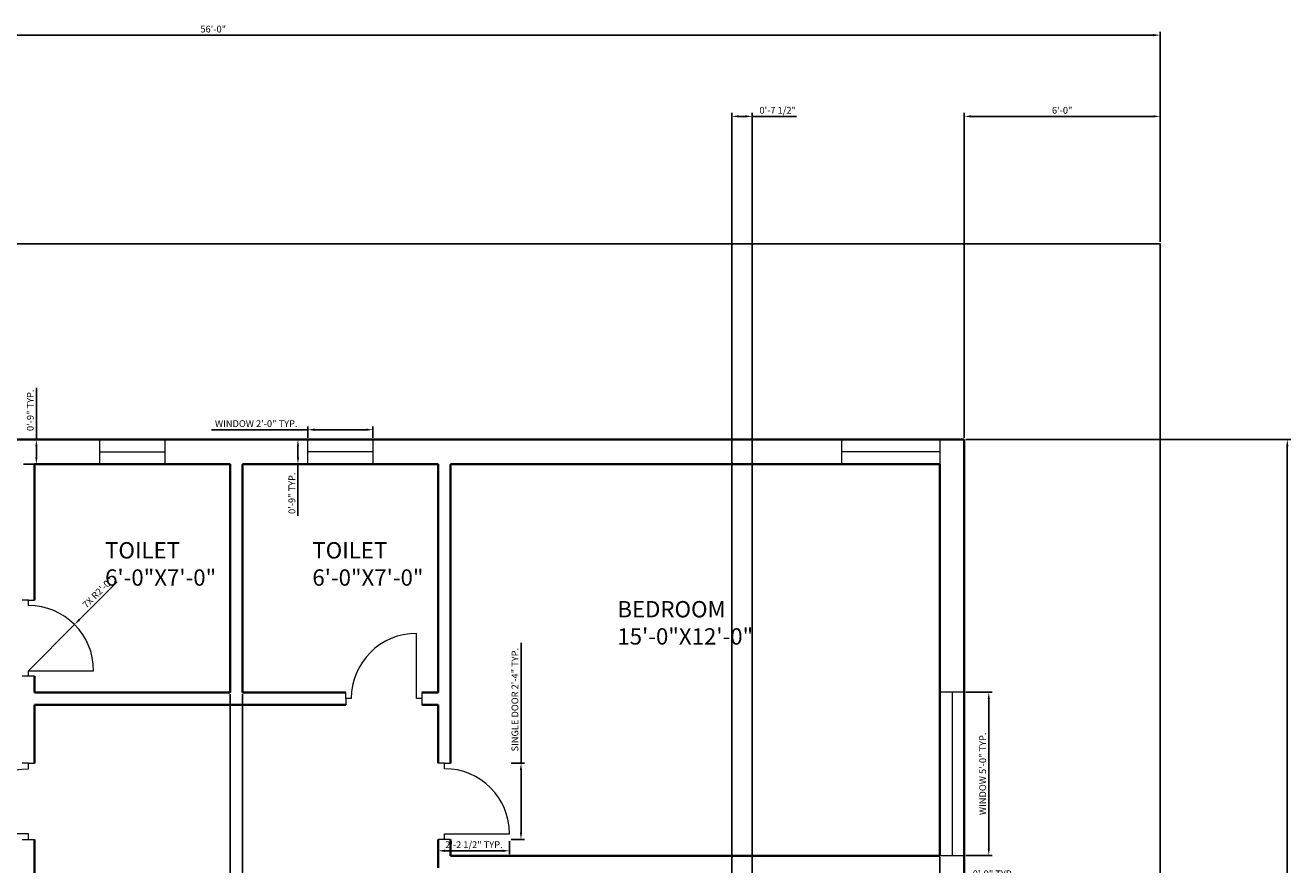
# Model space of a CAD drawing. Units: inches. Extents: x 3257 to 4085, y -12 to 956.
# Tile 6 of 6: x 3619 to 4085, y 648 to 956. Entities that reach past the tile are written whole.
import ezdxf

# ---------------------------------------------------------------- set-up
doc = ezdxf.new("R2010")
doc.units = ezdxf.units.IN
for name, color, linetype, lineweight in [('A-ANNO-DIMS', 2, 'Continuous', 18), ('A-AREA-IDEN', 7, 'Continuous', 18), ('A-DOOR', 3, 'Continuous', 18), ('A-GLAZ', 4, 'Continuous', 18), ('A-WALL', 7, 'Continuous', 35), ('C-PROP', 6, 'Continuous', 25)]:
    doc.layers.add(name, color=color, linetype=linetype, lineweight=lineweight)
doc.styles.get("Standard").update_dxf_attribs({"font": 'arial.ttf'})
doc.dimstyles.new('ISO-25', dxfattribs={"dimtxt": 2.5, "dimasz": 2.5, "dimexe": 1.25, "dimexo": 0.625, "dimtad": 1, "dimdec": 0, "dimlunit": 3, "dimtxsty": 'Standard', "dimcen": 2.5, "dimadec": 0, "dimazin": 0, "dimtfac": 1, "dimtdec": 0, "dimtmove": 0, "dimatfit": 3, "dimfxl": 1, "dimarcsym": 0})

# ---------------------------------------------------------------- blocks, each defined once
blk = doc.blocks.new('*D1')
at = {"layer": 'A-ANNO-DIMS', "color": 0, "lineweight": -2, "transparency": 16777216}
for p, q in [((3339.97, 876.63), (3339.97, 953.92)), ((3342.47, 952.67), (4033.97, 952.67)), ((4036.47, 876.63), (4036.47, 953.92))]:
    blk.add_line(p, q, dxfattribs=at)
at = {"layer": 'A-ANNO-DIMS', "color": 0, "transparency": 16777216}
for points in [[(3342.47, 953.09), (3342.47, 952.25), (3339.97, 952.67)], [(4033.97, 953.09), (4033.97, 952.25), (4036.47, 952.67)]]:
    blk.add_solid(points, dxfattribs=at)
at = {"layer": 'Defpoints', "color": 0, "transparency": 16777216}
for p in [(4036.47, 952.67), (3339.97, 876), (4036.47, 876)]:
    blk.add_point(p, dxfattribs=at)
at = {"layer": 'A-ANNO-DIMS', "color": 0, "transparency": 16777216, "insert": (3688.22, 954.57), "char_height": 2.5, "attachment_point": 5}
blk.add_mtext('56\'-0"', dxfattribs=at)
blk = doc.blocks.new('DOOR-SGL-24IN')
for p, q in [((2.25, 28), (0, 28)), ((2.25, 26), (2.25, 28)), ((2.25, 28), (4.5, 28)), ((2.25, 0), (2.25, 2)), ((2.25, 2), (26.25, 2)), ((4.5, 0), (0, 0))]:
    blk.add_line(p, q)
blk.add_arc((2.25, 2), 24, 0, 90)
blk = doc.blocks.new('WIN-36IN')
for p, q in [((0, 9), (36, 9)), ((0, 0), (0, 9)), ((36, 9), (36, 0)), ((0, 4.5), (36, 4.5)), ((36, 0), (0, 0))]:
    blk.add_line(p, q)
blk = doc.blocks.new('WIN-24IN')
for p, q in [((0, 9), (24, 9)), ((0, 0), (0, 9)), ((24, 9), (24, 0)), ((0, 4.5), (24, 4.5)), ((24, 0), (0, 0))]:
    blk.add_line(p, q)
blk = doc.blocks.new('WIN-60IN')
for p, q in [((0, 60), (0, 0)), ((9, 60), (0, 60)), ((4.5, 60), (4.5, 0)), ((9, 0), (9, 60)), ((0, 0), (9, 0))]:
    blk.add_line(p, q)
blk = doc.blocks.new('*D8')
at = {"layer": 'A-ANNO-DIMS', "color": 0, "lineweight": -2, "transparency": 16777216}
for p, q in [((3801.42, 685), (3801.42, 729.21)), ((3797.84, 685), (3802.67, 685)), ((3801.42, 659.5), (3801.42, 682.5)), ((3797.84, 657), (3802.67, 657))]:
    blk.add_line(p, q, dxfattribs=at)
at = {"layer": 'A-ANNO-DIMS', "color": 0, "transparency": 16777216}
for points in [[(3801, 682.5), (3801.83, 682.5), (3801.42, 685)], [(3801, 659.5), (3801.83, 659.5), (3801.42, 657)]]:
    blk.add_solid(points, dxfattribs=at)
at = {"layer": 'Defpoints', "color": 0, "transparency": 16777216}
for p in [(3797.22, 685), (3801.42, 685), (3797.22, 657)]:
    blk.add_point(p, dxfattribs=at)
at = {"layer": 'A-ANNO-DIMS', "color": 0, "transparency": 16777216, "insert": (3799.5, 708.36), "char_height": 2.5, "attachment_point": 5, "rotation": 90}
blk.add_mtext('SINGLE DOOR 2\'-4" TYP.', dxfattribs=at)
blk = doc.blocks.new('*D9')
at = {"layer": 'A-ANNO-DIMS', "color": 0, "lineweight": -2, "transparency": 16777216}
for p, q in [((3770.97, 656.38), (3770.97, 651.55)), ((3797.22, 656.38), (3797.22, 651.55)), ((3773.47, 652.8), (3794.72, 652.8))]:
    blk.add_line(p, q, dxfattribs=at)
at = {"layer": 'A-ANNO-DIMS', "color": 0, "transparency": 16777216}
for points in [[(3773.47, 653.22), (3773.47, 652.39), (3770.97, 652.8)], [(3794.72, 653.22), (3794.72, 652.39), (3797.22, 652.8)]]:
    blk.add_solid(points, dxfattribs=at)
at = {"layer": 'Defpoints', "color": 0, "transparency": 16777216}
for p in [(3770.97, 657), (3797.22, 657), (3797.22, 652.8)]:
    blk.add_point(p, dxfattribs=at)
at = {"layer": 'A-ANNO-DIMS', "color": 0, "transparency": 16777216, "insert": (3784.09, 654.72), "char_height": 2.5, "attachment_point": 5}
blk.add_mtext('2\'-2 1/2" TYP.', dxfattribs=at)
blk = doc.blocks.new('*D13')
at = {"layer": 'A-ANNO-DIMS', "color": 0, "lineweight": -2, "transparency": 16777216}
for p, q in [((3623.17, 804), (3623.17, 822.99)), ((3618.39, 804), (3624.42, 804)), ((3623.17, 797.5), (3623.17, 801.5)), ((3618.39, 795), (3624.42, 795))]:
    blk.add_line(p, q, dxfattribs=at)
at = {"layer": 'A-ANNO-DIMS', "color": 0, "transparency": 16777216}
for points in [[(3622.75, 801.5), (3623.58, 801.5), (3623.17, 804)], [(3622.75, 797.5), (3623.58, 797.5), (3623.17, 795)]]:
    blk.add_solid(points, dxfattribs=at)
at = {"layer": 'Defpoints', "color": 0, "transparency": 16777216}
for p in [(3617.77, 804), (3623.17, 804), (3617.77, 795)]:
    blk.add_point(p, dxfattribs=at)
at = {"layer": 'A-ANNO-DIMS', "color": 0, "transparency": 16777216, "insert": (3621.26, 814.75), "char_height": 2.5, "attachment_point": 5, "rotation": 90}
blk.add_mtext('0\'-9" TYP.', dxfattribs=at)
blk = doc.blocks.new('*D14')
at = {"layer": 'A-ANNO-DIMS', "color": 0, "lineweight": -2, "transparency": 16777216}
for p, q in [((3722.97, 807.6), (3687.58, 807.6)), ((3722.97, 804.63), (3722.97, 808.85)), ((3744.47, 807.6), (3725.47, 807.6)), ((3746.97, 804.63), (3746.97, 808.85))]:
    blk.add_line(p, q, dxfattribs=at)
at = {"layer": 'A-ANNO-DIMS', "color": 0, "transparency": 16777216}
for points in [[(3725.47, 808.02), (3725.47, 807.19), (3722.97, 807.6)], [(3744.47, 808.02), (3744.47, 807.19), (3746.97, 807.6)]]:
    blk.add_solid(points, dxfattribs=at)
at = {"layer": 'Defpoints', "color": 0, "transparency": 16777216}
for p in [(3722.97, 807.6), (3722.97, 804), (3746.97, 804)]:
    blk.add_point(p, dxfattribs=at)
at = {"layer": 'A-ANNO-DIMS', "color": 0, "transparency": 16777216, "insert": (3704.03, 809.52), "char_height": 2.5, "attachment_point": 5}
blk.add_mtext('WINDOW 2\'-0" TYP.', dxfattribs=at)
blk = doc.blocks.new('*D15')
at = {"layer": 'A-ANNO-DIMS', "color": 0, "lineweight": -2, "transparency": 16777216}
for p, q in [((3722.34, 804), (3718.12, 804)), ((3719.37, 801.5), (3719.37, 797.5)), ((3722.34, 795), (3718.12, 795)), ((3719.37, 795), (3719.37, 776.01))]:
    blk.add_line(p, q, dxfattribs=at)
at = {"layer": 'A-ANNO-DIMS', "color": 0, "transparency": 16777216}
for points in [[(3718.95, 801.5), (3719.78, 801.5), (3719.37, 804)], [(3718.95, 797.5), (3719.78, 797.5), (3719.37, 795)]]:
    blk.add_solid(points, dxfattribs=at)
at = {"layer": 'Defpoints', "color": 0, "transparency": 16777216}
for p in [(3722.97, 804), (3719.37, 795), (3722.97, 795)]:
    blk.add_point(p, dxfattribs=at)
at = {"layer": 'A-ANNO-DIMS', "color": 0, "transparency": 16777216, "insert": (3717.47, 784.26), "char_height": 2.5, "attachment_point": 5, "rotation": 90}
blk.add_mtext('0\'-9" TYP.', dxfattribs=at)
blk = doc.blocks.new('*D16')
at = {"layer": 'A-ANNO-DIMS', "color": 0, "lineweight": -2, "transparency": 16777216}
for p, q in [((3965.09, 711.11), (3974.72, 711.11)), ((3973.47, 653.61), (3973.47, 708.61)), ((3965.09, 651.11), (3974.72, 651.11))]:
    blk.add_line(p, q, dxfattribs=at)
at = {"layer": 'A-ANNO-DIMS', "color": 0, "transparency": 16777216}
for points in [[(3973.05, 708.61), (3973.88, 708.61), (3973.47, 711.11)], [(3973.05, 653.61), (3973.88, 653.61), (3973.47, 651.11)]]:
    blk.add_solid(points, dxfattribs=at)
at = {"layer": 'Defpoints', "color": 0, "transparency": 16777216}
for p in [(3964.47, 711.11), (3973.47, 711.11), (3964.47, 651.11)]:
    blk.add_point(p, dxfattribs=at)
at = {"layer": 'A-ANNO-DIMS', "color": 0, "transparency": 16777216, "insert": (3971.55, 681.11), "char_height": 2.5, "attachment_point": 5, "rotation": 90}
blk.add_mtext('WINDOW 5\'-0" TYP.', dxfattribs=at)
blk = doc.blocks.new('*D17')
at = {"layer": 'A-ANNO-DIMS', "color": 0, "lineweight": -2, "transparency": 16777216}
for p, q in [((3955.47, 650.49), (3955.47, 640.86)), ((3964.47, 650.49), (3964.47, 640.86)), ((3957.97, 642.11), (3961.97, 642.11)), ((3964.47, 642.11), (3983.46, 642.11))]:
    blk.add_line(p, q, dxfattribs=at)
at = {"layer": 'A-ANNO-DIMS', "color": 0, "transparency": 16777216}
for points in [[(3957.97, 642.53), (3957.97, 641.69), (3955.47, 642.11)], [(3961.97, 642.53), (3961.97, 641.69), (3964.47, 642.11)]]:
    blk.add_solid(points, dxfattribs=at)
at = {"layer": 'Defpoints', "color": 0, "transparency": 16777216}
for p in [(3955.47, 651.11), (3964.47, 651.11), (3964.47, 642.11)]:
    blk.add_point(p, dxfattribs=at)
at = {"layer": 'A-ANNO-DIMS', "color": 0, "transparency": 16777216, "insert": (3975.21, 644.01), "char_height": 2.5, "attachment_point": 5}
blk.add_mtext('0\'-9" TYP.', dxfattribs=at)
blk = doc.blocks.new('*D19')
at = {"layer": 'A-ANNO-DIMS', "color": 0, "lineweight": -2, "transparency": 16777216}
for p, q in [((3965.09, 804), (4084.52, 804)), ((4083.27, 159.5), (4083.27, 801.5)), ((3965.09, 157), (4084.52, 157))]:
    blk.add_line(p, q, dxfattribs=at)
at = {"layer": 'A-ANNO-DIMS', "color": 0, "transparency": 16777216}
for points in [[(4082.85, 801.5), (4083.68, 801.5), (4083.27, 804)], [(4082.85, 159.5), (4083.68, 159.5), (4083.27, 157)]]:
    blk.add_solid(points, dxfattribs=at)
at = {"layer": 'Defpoints', "color": 0, "transparency": 16777216}
for p in [(3964.47, 804), (4083.27, 804), (3964.47, 157)]:
    blk.add_point(p, dxfattribs=at)
at = {"layer": 'A-ANNO-DIMS', "color": 0, "transparency": 16777216, "insert": (4081.37, 480.5), "char_height": 2.5, "attachment_point": 5, "rotation": 90}
blk.add_mtext('53\'-11"', dxfattribs=at)
blk = doc.blocks.new('*D20')
at = {"layer": 'A-ANNO-DIMS', "color": 0, "lineweight": -2, "transparency": 16777216}
for p, q in [((3964.47, 804.63), (3964.47, 924.05)), ((3966.97, 922.8), (4033.97, 922.8)), ((4036.47, 876.63), (4036.47, 924.05))]:
    blk.add_line(p, q, dxfattribs=at)
at = {"layer": 'A-ANNO-DIMS', "color": 0, "transparency": 16777216}
for points in [[(3966.97, 923.22), (3966.97, 922.39), (3964.47, 922.8)], [(4033.97, 923.22), (4033.97, 922.39), (4036.47, 922.8)]]:
    blk.add_solid(points, dxfattribs=at)
at = {"layer": 'Defpoints', "color": 0, "transparency": 16777216}
for p in [(4036.47, 922.8), (4036.47, 876), (3964.47, 804)]:
    blk.add_point(p, dxfattribs=at)
at = {"layer": 'A-ANNO-DIMS', "color": 0, "transparency": 16777216, "insert": (4000.47, 924.7), "char_height": 2.5, "attachment_point": 5}
blk.add_mtext('6\'-0"', dxfattribs=at)
blk = doc.blocks.new('*D25')
at = {"layer": 'A-ANNO-DIMS', "color": 0, "lineweight": -2, "transparency": 16777216}
for p, q in [((3878.97, 441.13), (3878.97, 924.05)), ((3881.47, 922.8), (3883.97, 922.8)), ((3886.47, 441.13), (3886.47, 924.05)), ((3886.47, 922.8), (3902.69, 922.8))]:
    blk.add_line(p, q, dxfattribs=at)
at = {"layer": 'A-ANNO-DIMS', "color": 0, "transparency": 16777216}
for points in [[(3881.47, 923.22), (3881.47, 922.39), (3878.97, 922.8)], [(3883.97, 923.22), (3883.97, 922.39), (3886.47, 922.8)]]:
    blk.add_solid(points, dxfattribs=at)
at = {"layer": 'Defpoints', "color": 0, "transparency": 16777216}
for p in [(3886.47, 922.8), (3878.97, 440.5), (3886.47, 440.5)]:
    blk.add_point(p, dxfattribs=at)
at = {"layer": 'A-ANNO-DIMS', "color": 0, "transparency": 16777216, "insert": (3895.83, 924.72), "char_height": 2.5, "attachment_point": 5}
blk.add_mtext('0\'-7 1/2"', dxfattribs=at)
blk = doc.blocks.new('*D26')
at = {"layer": 'A-ANNO-DIMS', "color": 0, "lineweight": -2, "transparency": 16777216}
for p, q in [((3694.47, 710.38), (3694.47, -11.05)), ((3698.97, 710.38), (3698.97, -11.05)), ((3691.97, -9.8), (3689.47, -9.8)), ((3694.47, -9.8), (3698.97, -9.8)), ((3701.47, -9.8), (3717.69, -9.8))]:
    blk.add_line(p, q, dxfattribs=at)
at = {"layer": 'A-ANNO-DIMS', "color": 0, "transparency": 16777216}
for points in [[(3691.97, -9.38), (3691.97, -10.21), (3694.47, -9.8)], [(3701.47, -9.38), (3701.47, -10.21), (3698.97, -9.8)]]:
    blk.add_solid(points, dxfattribs=at)
at = {"layer": 'Defpoints', "color": 0, "transparency": 16777216}
for p in [(3694.47, 711), (3698.97, 711), (3698.97, -9.8)]:
    blk.add_point(p, dxfattribs=at)
at = {"layer": 'A-ANNO-DIMS', "color": 0, "transparency": 16777216, "insert": (3710.83, -7.88), "char_height": 2.5, "attachment_point": 5}
blk.add_mtext('0\'-4 1/2"', dxfattribs=at)
blk = doc.blocks.new('*D27')
at = {"layer": 'A-ANNO-DIMS', "color": 0, "lineweight": -2, "transparency": 16777216}
for p, q in [((3652.9, 751.69), (3638.96, 737.74)), ((3620.22, 719), (3637.19, 735.97))]:
    blk.add_line(p, q, dxfattribs=at)
at = {"layer": 'A-ANNO-DIMS', "color": 0, "transparency": 16777216}
blk.add_solid([(3638.66, 738.04), (3639.25, 737.45), (3637.19, 735.97)], dxfattribs=at)
at = {"layer": 'Defpoints', "color": 0, "transparency": 16777216}
for p in [(3637.19, 735.97), (3620.22, 719)]:
    blk.add_point(p, dxfattribs=at)
at = {"layer": 'A-ANNO-DIMS', "color": 0, "transparency": 16777216, "insert": (3646.03, 747.5), "char_height": 2.5, "attachment_point": 5, "rotation": 44.9997}
blk.add_mtext('7X R2\'-0"', dxfattribs=at)

msp = doc.modelspace()

# ---------------------------------------------------------------- linework, layer by layer
at = {"layer": 'A-WALL'}
for p, q in [((3464.97, 804), (3928.47, 804)), ((3928.47, 804), (3964.47, 804)), ((3964.47, 804), (3964.47, 795)), ((3622.47, 795), (3622.47, 745)), ((3622.47, 795), (3694.47, 795)), ((3694.47, 795), (3694.47, 711)), ((3698.97, 795), (3698.97, 711)), ((3698.97, 795), (3770.97, 795)), ((3770.97, 795), (3770.97, 711)), ((3775.47, 795), (3775.47, 685)), ((3775.47, 795), (3919.47, 795)), ((3919.47, 795), (3955.47, 795)), ((3955.47, 795), (3955.47, 685)), ((3964.47, 795), (3964.47, 685)), ((3622.47, 717), (3622.47, 711)), ((3622.47, 711), (3694.47, 711)), ((3698.97, 711), (3736.97, 711)), ((3764.97, 711), (3770.97, 711)), ((3622.47, 706.5), (3694.47, 706.5)), ((3622.47, 706.5), (3622.47, 685)), ((3694.47, 706.5), (3698.97, 706.5)), ((3698.97, 706.5), (3736.97, 706.5)), ((3764.97, 706.5), (3770.97, 706.5)), ((3770.97, 706.5), (3770.97, 685)), ((3955.47, 685), (3955.47, 651)), ((3964.47, 685), (3964.47, 157)), ((3622.47, 657), (3622.47, 651)), ((3622.47, 657), (3622.47, 533.5)), ((3770.97, 657), (3770.97, 646.5)), ((3775.47, 657), (3775.47, 651)), ((3775.47, 651), (3955.47, 651))]:
    msp.add_line(p, q, dxfattribs=at)
at = {"layer": 'C-PROP'}
for p, q in [((3464.97, 876), (3928.47, 876)), ((4036.47, 876), (3928.47, 876)), ((4036.47, 795), (4036.47, 876)), ((4036.47, 795), (4036.47, 685)), ((4036.47, 685), (4036.47, 37))]:
    msp.add_line(p, q, dxfattribs=at)

# ---------------------------------------------------------------- block references
at = {"layer": 'A-DOOR'}
for p in [(3617.97, 717), (3770.97, 657)]:
    msp.add_blockref('DOOR-SGL-24IN', p, dxfattribs=at)
at = {"layer": 'A-DOOR', "rotation": 89.99999999999872}
msp.add_blockref('DOOR-SGL-24IN', (3764.97, 706.5), dxfattribs=at)
at = {"layer": 'A-DOOR', "extrusion": (0, 0, -1), "zscale": -1}
msp.add_blockref('DOOR-SGL-24IN', (-3622.47, 657), dxfattribs=at)
at = {"layer": 'A-GLAZ'}
for name, p in [('WIN-24IN', (3646.47, 795)), ('WIN-60IN', (3955.47, 651.11))]:
    msp.add_blockref(name, p, dxfattribs=at)
at = {"layer": 'A-GLAZ', "rotation": 180}
for name, p in [('WIN-24IN', (3746.97, 804)), ('WIN-36IN', (3955.47, 804))]:
    msp.add_blockref(name, p, dxfattribs=at)

# ---------------------------------------------------------------- texts
at = {"layer": 'A-AREA-IDEN', "char_height": 6, "attachment_point": 1}
for s, insert in [('TOILET\\P6\'-0"X7\'-0" ', (3648.44, 766.27)), ('TOILET\\P6\'-0"X7\'-0" ', (3724.68, 766.27)), ('BEDROOM\\P15\'-0"X12\'-0"', (3836.86, 744.62))]:
    msp.add_mtext(s, dxfattribs=dict(at, insert=insert))

# ---------------------------------------------------------------- dimensions: what is measured, and where the dimension line sits
at = {"layer": 'A-ANNO-DIMS'}
for base, p1, p2, text, override, picture, middle in [((4036.47, 952.67), (3339.97, 876), (4036.47, 876), '56\'-0"', {"dimclrd": 0, "dimclre": 0, "dimclrt": 0}, '*D1', (3688.22, 954.57)), ((3797.21772149, 652.80291232), (3770.96772149, 657.00291232), (3797.21772149, 657.00291232), '<> TYP.', {"dimdec": 1, "dimlfac": 1, "dimrnd": 0, "dimzin": 1, "dimdsep": 46, "dimlunit": 4, "dimfrac": 2}, '*D9', (3784.09272149, 654.72054533)), ((3964.47, 642.11), (3955.47, 651.11), (3964.47, 651.11), '<> TYP.', {"dimdec": 1, "dimlfac": 1, "dimrnd": 0, "dimzin": 1, "dimdsep": 46, "dimlunit": 4, "dimfrac": 2}, '*D17', (3975.21, 644.01))]:
    dim = msp.add_linear_dim(base=base, p1=p1, p2=p2, text=text, dimstyle='ISO-25', override=override, dxfattribs=at)
    dim.commit()
    dim.dimension.update_dxf_attribs({"geometry": picture, "text_midpoint": middle})
for base, p1, p2, picture, middle in [((3886.47, 922.8), (3878.97, 440.5), (3886.47, 440.5), '*D25', (3895.83, 924.72)), ((4036.47, 922.8), (3964.47, 804), (4036.47, 876), '*D20', (4000.47, 924.7)), ((3698.97, -9.8), (3694.47, 711), (3698.97, 711), '*D26', (3710.83, -7.88))]:
    dim = msp.add_linear_dim(base=base, p1=p1, p2=p2, dimstyle='ISO-25', override={"dimdec": 1, "dimlfac": 1, "dimrnd": 0, "dimzin": 1, "dimdsep": 46, "dimlunit": 4, "dimfrac": 2}, dxfattribs=at)
    dim.commit()
    dim.dimension.update_dxf_attribs({"geometry": picture, "text_midpoint": middle})
for base, p1, p2, angle, text, picture, middle in [((3623.17, 804), (3617.77, 795), (3617.77, 804), 90, '<> TYP.', '*D13', (3621.26, 814.75)), ((3722.97, 807.6), (3746.97, 804), (3722.97, 804), 180, 'WINDOW <> TYP.', '*D14', (3704.03, 809.52)), ((3719.37, 795), (3722.97, 804), (3722.97, 795), 270, '<> TYP.', '*D15', (3717.47, 784.26)), ((3801.42, 685), (3797.22, 657), (3797.22, 685), 90, 'SINGLE DOOR <> TYP.', '*D8', (3799.5, 708.36)), ((3973.47, 711.11), (3964.47, 651.11), (3964.47, 711.11), 90, 'WINDOW <> TYP.', '*D16', (3971.55, 681.11))]:
    dim = msp.add_linear_dim(base=base, p1=p1, p2=p2, angle=angle, text=text, dimstyle='ISO-25', override={"dimdec": 1, "dimlfac": 1, "dimrnd": 0, "dimzin": 1, "dimdsep": 46, "dimlunit": 4, "dimfrac": 2}, dxfattribs=at)
    dim.commit()
    dim.dimension.update_dxf_attribs({"geometry": picture, "text_midpoint": middle})
dim = msp.add_linear_dim(base=(4083.27, 804), p1=(3964.47, 157), p2=(3964.47, 804), angle=90, dimstyle='ISO-25', override={"dimdec": 1, "dimlfac": 1, "dimrnd": 0, "dimzin": 1, "dimdsep": 46, "dimlunit": 4, "dimfrac": 2}, dxfattribs=at)
dim.commit()
dim.dimension.update_dxf_attribs({"geometry": '*D19', "text_midpoint": (4081.37, 480.5)})
dim = msp.add_radius_dim(center=(3620.22, 719), mpoint=(3637.19, 735.97), text='7X <>', dimstyle='ISO-25', override={"dimdec": 1, "dimlfac": 1, "dimrnd": 0, "dimzin": 1, "dimdsep": 46, "dimlunit": 4, "dimfrac": 2}, dxfattribs=at)
dim.commit()
dim.dimension.update_dxf_attribs({"geometry": '*D27', "text_midpoint": (3647.37, 746.16), "dimtype": 164})

doc.saveas('drawing.dxf')
